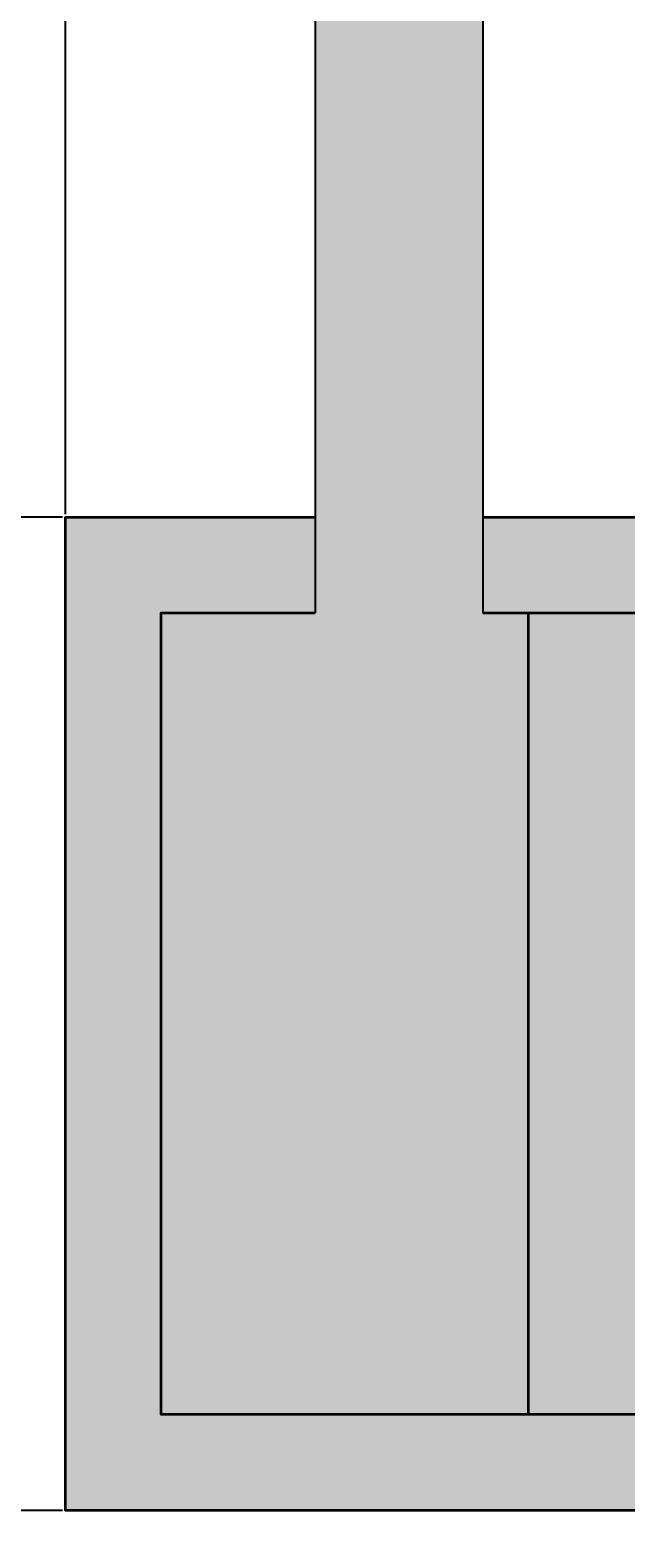
# Model space of a CAD drawing. Units: millimetres. Extents: x -11 to 280, y -4 to 208.
# Tile 26 of 55: x 150 to 163, y 22 to 54. Entities that reach past the tile are written whole.
import ezdxf

# ---------------------------------------------------------------- set-up
doc = ezdxf.new("R2010")
doc.units = ezdxf.units.MM
for name, color, linetype, lineweight in [('M-DIMS', 2, 'Continuous', 18), ('M-HYDR-CYL', 7, 'Continuous', 35), ('M-HYDR-CYL-PATT', 252, 'Continuous', 13), ('M-HYDR-RETN', 7, 'Continuous', 25)]:
    doc.layers.add(name, color=color, linetype=linetype, lineweight=lineweight)
doc.layers.add('M-HYDR-RETN-PATT', color=114, linetype='Continuous', lineweight=13, true_color=0x139b48)
doc.styles.get("Standard").update_dxf_attribs({"font": 'arial.ttf'})
doc.dimstyles.get("Standard").update_dxf_attribs({"dimtxt": 0.18, "dimasz": 0.18, "dimexe": 0.18, "dimexo": 0.0625, "dimgap": 0.09, "dimtad": 0, "dimtih": 1, "dimtoh": 1, "dimdec": 4, "dimzin": 0, "dimdsep": 46, "dimtxsty": 'Standard', "dimcen": 0.09, "dimadec": 0, "dimazin": 0, "dimtfac": 1, "dimtdec": 4, "dimtofl": 0, "dimtmove": 0, "dimatfit": 3, "dimfxl": 1, "dimtolj": 1, "dimtzin": 0, "dimarcsym": 0})

# ---------------------------------------------------------------- blocks, each defined once
blk = doc.blocks.new('*D4')
at = {"layer": 'Defpoints', "color": 0, "transparency": 16777216}
for p in [(4.763, 84.426), (266.035, 51.733), (266.035, -3.415)]:
    blk.add_point(p, dxfattribs=at)
at = {"layer": 'M-DIMS', "color": 0, "lineweight": -2, "transparency": 16777216}
for p, q in [((4.763, 84.364), (4.763, -3.595)), ((266.035, 51.67), (266.035, -3.595)), ((4.943, -3.415), (134.934, -3.415)), ((265.855, -3.415), (135.864, -3.415))]:
    blk.add_line(p, q, dxfattribs=at)
at = {"layer": 'M-DIMS', "color": 0, "transparency": 16777216}
for points in [[(4.943, -3.385), (4.943, -3.445), (4.763, -3.415)], [(265.855, -3.385), (265.855, -3.445), (266.035, -3.415)]]:
    blk.add_solid(points, dxfattribs=at)
at = {"layer": 'M-DIMS', "color": 0, "transparency": 16777216, "insert": (135.399, -3.415), "char_height": 0.18, "attachment_point": 5}
blk.add_mtext('\\A1;261.27', dxfattribs=at)
blk = doc.blocks.new('*D5')
at = {"layer": 'Defpoints', "color": 0, "transparency": 16777216}
for p in [(24.759, 192.645), (-10.087, 11.435), (261.686, 11.435)]:
    blk.add_point(p, dxfattribs=at)
at = {"layer": 'M-DIMS', "color": 0, "lineweight": -2, "transparency": 16777216}
for p, q in [((24.696, 192.645), (-10.267, 192.645)), ((-10.087, 192.465), (-10.087, 102.222)), ((-10.087, 11.615), (-10.087, 101.858)), ((261.624, 11.435), (-10.267, 11.435))]:
    blk.add_line(p, q, dxfattribs=at)
at = {"layer": 'M-DIMS', "color": 0, "transparency": 16777216}
for points in [[(-10.117, 192.465), (-10.057, 192.465), (-10.087, 192.645)], [(-10.117, 11.615), (-10.057, 11.615), (-10.087, 11.435)]]:
    blk.add_solid(points, dxfattribs=at)
at = {"layer": 'M-DIMS', "color": 0, "transparency": 16777216, "insert": (-10.087, 102.04), "char_height": 0.18, "attachment_point": 5}
blk.add_mtext('\\A1;181.2', dxfattribs=at)
blk = doc.blocks.new('*D18')
at = {"layer": 'Defpoints', "color": 0, "transparency": 16777216}
for p in [(173.804, 207.495), (173.804, 65.064), (151.022, 43.599)]:
    blk.add_point(p, dxfattribs=at)
at = {"layer": 'M-DIMS', "color": 0, "lineweight": -2, "transparency": 16777216}
for p, q in [((151.022, 43.662), (151.022, 207.675)), ((173.804, 65.126), (173.804, 207.675)), ((151.202, 207.495), (162.017, 207.495)), ((173.624, 207.495), (162.808, 207.495))]:
    blk.add_line(p, q, dxfattribs=at)
at = {"layer": 'M-DIMS', "color": 0, "transparency": 16777216}
for points in [[(151.202, 207.525), (151.202, 207.465), (151.022, 207.495)], [(173.624, 207.525), (173.624, 207.465), (173.804, 207.495)]]:
    blk.add_solid(points, dxfattribs=at)
at = {"layer": 'M-DIMS', "color": 0, "transparency": 16777216, "insert": (162.413, 207.495), "char_height": 0.18, "attachment_point": 5}
blk.add_mtext('\\A1;22.78', dxfattribs=at)
blk = doc.blocks.new('*D20')
at = {"layer": 'Defpoints', "color": 0, "transparency": 16777216}
for p in [(231.68, 207.495), (151.022, 43.599), (231.68, 43.599)]:
    blk.add_point(p, dxfattribs=at)
at = {"layer": 'M-DIMS', "color": 0, "lineweight": -2, "transparency": 16777216}
for p, q in [((151.022, 43.662), (151.022, 207.675)), ((231.68, 43.662), (231.68, 207.675)), ((151.202, 207.495), (190.957, 207.495)), ((231.5, 207.495), (191.745, 207.495))]:
    blk.add_line(p, q, dxfattribs=at)
at = {"layer": 'M-DIMS', "color": 0, "transparency": 16777216}
for points in [[(151.202, 207.525), (151.202, 207.465), (151.022, 207.495)], [(231.5, 207.525), (231.5, 207.465), (231.68, 207.495)]]:
    blk.add_solid(points, dxfattribs=at)
at = {"layer": 'M-DIMS', "color": 0, "transparency": 16777216, "insert": (191.351, 207.495), "char_height": 0.18, "attachment_point": 5}
blk.add_mtext('\\A1;80.66', dxfattribs=at)
blk = doc.blocks.new('*D21')
at = {"layer": 'Defpoints', "color": 0, "transparency": 16777216}
for p in [(136.172, 43.599), (151.022, 43.599), (151.022, 22.846)]:
    blk.add_point(p, dxfattribs=at)
at = {"layer": 'M-DIMS', "color": 0, "lineweight": -2, "transparency": 16777216}
for p, q in [((150.959, 43.599), (135.992, 43.599)), ((136.172, 43.419), (136.172, 33.405)), ((136.172, 23.026), (136.172, 33.041)), ((150.959, 22.846), (135.992, 22.846))]:
    blk.add_line(p, q, dxfattribs=at)
at = {"layer": 'M-DIMS', "color": 0, "transparency": 16777216}
for points in [[(136.142, 43.419), (136.202, 43.419), (136.172, 43.599)], [(136.142, 23.026), (136.202, 23.026), (136.172, 22.846)]]:
    blk.add_solid(points, dxfattribs=at)
at = {"layer": 'M-DIMS', "color": 0, "transparency": 16777216, "insert": (136.172, 33.223), "char_height": 0.18, "attachment_point": 5}
blk.add_mtext('\\A1;20.753', dxfattribs=at)

msp = doc.modelspace()

# ---------------------------------------------------------------- hatches: boundary and pattern name
at = {"layer": 'M-HYDR-CYL-PATT'}
h = msp.add_hatch(color=256, dxfattribs=at)
h.set_gradient(color1=(128, 128, 128), color2=(99, 100, 102), tint=1)
h.paths.add_polyline_path([(163.0955, 41.5991), (160.6935, 41.5991), (160.6935, 24.846), (163.0955, 24.846)])
h.paths.add_polyline_path([(259.871, 34.7226), (163.0955, 34.7226), (163.0955, 31.7226), (259.871, 31.7226, 1)])
h.paths.add_polyline_path([(257.0171, 42.0966), (265.5958, 50.6754, 1), (263.4745, 52.7967), (253.6316, 42.9537), (253.6316, 34.7226), (257.0171, 34.7226)])
h.paths.add_polyline_path([(257.0171, 25.6028), (257.0171, 31.7226), (253.6316, 31.7226), (253.6316, 26.785), (249.6456, 22.7991), (249.6456, 13.7204, 1), (252.6456, 13.7204), (252.6456, 21.2313)])
h.paths.add_polyline_path([(265.4334, 20.9382), (261.6863, 20.9382), (261.6863, 11.4346), (265.4334, 11.4346)])
h.paths.add_polyline_path([(261.6863, 17.1598), (252.6456, 17.1598), (252.6456, 15.9126), (261.6863, 15.9126)])
h = msp.add_hatch(color=256, dxfattribs=at)
h.set_gradient(color1=(102, 52, 60), color2=(102, 52, 60), tint=1)
h.paths.add_polyline_path([(153.0217, 24.846), (153.0217, 41.5991), (156.2446, 41.5991), (156.2446, 43.5991), (151.0217, 43.5991), (151.0217, 22.846), (231.6803, 22.846), (231.6803, 31.7226), (229.6803, 31.7226), (229.6803, 24.846)])
h.paths.add_polyline_path([(159.7446, 43.5991), (159.7446, 41.5991), (163.0955, 41.5991), (229.6803, 41.5991), (229.6803, 34.7226), (231.6803, 34.7226), (231.6803, 43.5991)], flags=17)
at = {"layer": 'M-HYDR-RETN-PATT'}
h = msp.add_hatch(color=256, dxfattribs=at)
h.set_gradient(color1=(19, 155, 72), color2=(19, 155, 72), tint=1)
h.paths.add_polyline_path([(17.9701, 159.0814), (29.2015, 159.0814), (29.2015, 162.5814), (14.4701, 162.5814), (14.4701, 98.0213), (17.9701, 98.0213)])
h.paths.add_polyline_path([(17.9701, 84.4261), (14.4701, 84.4261), (14.4701, 54.3099), (156.2446, 54.3099), (156.2446, 57.8099), (17.9701, 57.8099)])
h.paths.add_polyline_path([(120.5137, 74.3991), (17.9701, 74.3991), (17.9701, 70.8991), (120.5137, 70.8991)], flags=17)
h.paths.add_polyline_path([(184.7092, 75.04, 0.4142136), (179.7092, 80.04), (156.2446, 80.04), (156.2446, 57.8099), (156.2446, 54.3099), (156.2446, 43.5991), (159.7446, 43.5991), (159.7446, 57.8099), (159.7446, 76.54), (176.2092, 76.54, -0.4142136), (181.2092, 71.54), (181.2092, 57.8099), (159.7446, 57.8099), (159.7446, 54.3099), (184.7092, 54.3099)])
h = msp.add_hatch(color=256, dxfattribs=at)
h.set_gradient(color1=(19, 155, 72), color2=(19, 155, 72), tint=1)
h.paths.add_polyline_path([(160.6935, 41.5991), (159.7446, 41.5991), (159.7446, 43.5991), (156.2446, 43.5991), (156.2446, 41.5991), (154.7803, 41.5991), (154.7803, 24.846), (160.6935, 24.846)])
h = msp.add_hatch(color=256, dxfattribs=at)
h.set_gradient(color1=(19, 155, 72), color2=(19, 155, 72), tint=1)
h.paths.add_polyline_path([(154.7803, 41.5991), (153.0217, 41.5991), (153.0217, 24.846), (154.7803, 24.846)])

# ---------------------------------------------------------------- linework, layer by layer
at = {"layer": 'M-HYDR-CYL'}
msp.add_line((160.6935, 41.5991), (160.6935, 24.846), dxfattribs=at)
for points in [[(231.6803, 31.7226), (231.6803, 22.846), (151.0217, 22.846), (151.0217, 43.5991), (156.2446, 43.5991)], [(159.7446, 43.5991), (231.6803, 43.5991), (231.6803, 34.7226)], [(229.6803, 31.7226), (229.6803, 24.846), (153.0217, 24.846), (153.0217, 41.5991), (156.2446, 41.5991)], [(159.7446, 41.5991), (163.0955, 41.5991), (163.0955, 24.846), (154.7803, 24.846)], [(154.7803, 41.5991), (156.2446, 41.5991)], [(159.7446, 41.5991), (229.6803, 41.5991), (229.6803, 34.7226)]]:
    msp.add_lwpolyline(points, dxfattribs=at)
at = {"layer": 'M-HYDR-RETN'}
for points in [[(156.2446, 57.8099), (156.2446, 41.5991)], [(159.7446, 57.8099), (159.7446, 41.5991)]]:
    msp.add_lwpolyline(points, dxfattribs=at)

# ---------------------------------------------------------------- dimensions: what is measured, and where the dimension line sits
at = {"layer": 'M-DIMS'}
for base, p1, p2, picture, middle in [((173.8038, 207.495), (151.0217, 43.5991), (173.8038, 65.0638), '*D18', (162.4127, 207.495)), ((231.6803, 207.495), (151.0217, 43.5991), (231.6803, 43.5991), '*D20', (191.351, 207.495)), ((266.0352, -3.4154), (4.7635, 84.4261), (266.0352, 51.7328), '*D4', (135.3993, -3.4154))]:
    dim = msp.add_linear_dim(base=base, p1=p1, p2=p2, dimstyle='Standard', override={"dimdec": 2, "dimlfac": 1, "dimrnd": 0, "dimzin": 0, "dimdsep": 46, "dimlunit": 2}, dxfattribs=at)
    dim.commit()
    dim.dimension.update_dxf_attribs({"geometry": picture, "text_midpoint": middle})
for base, p1, p2, override, picture, middle in [((-10.0865, 11.4346), (24.7588, 192.645), (261.6863, 11.4346), {"dimdec": 1, "dimlfac": 1, "dimrnd": 0, "dimzin": 0, "dimdsep": 46, "dimlunit": 2}, '*D5', (-10.0865, 102.0398)), ((136.1717, 43.5991), (151.0217, 22.846), (151.0217, 43.5991), {"dimdec": 3, "dimlfac": 1, "dimrnd": 0, "dimzin": 0, "dimdsep": 46, "dimlunit": 2}, '*D21', (136.1717, 33.2226))]:
    dim = msp.add_linear_dim(base=base, p1=p1, p2=p2, angle=90, dimstyle='Standard', override=override, dxfattribs=at)
    dim.commit()
    dim.dimension.update_dxf_attribs({"geometry": picture, "text_midpoint": middle})

doc.saveas('drawing.dxf')
